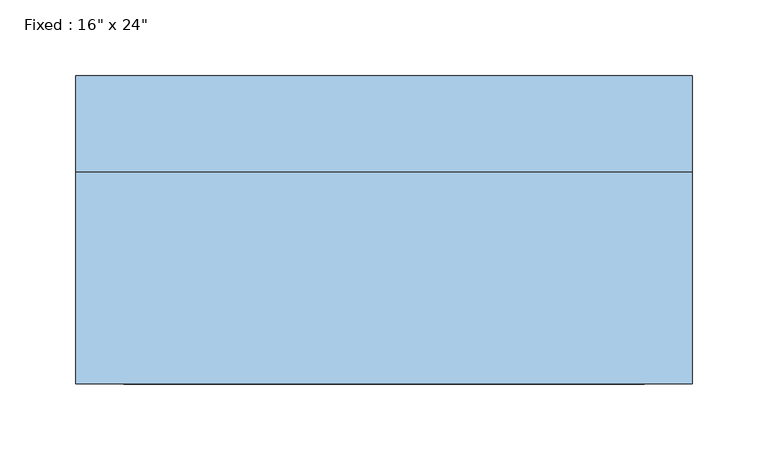
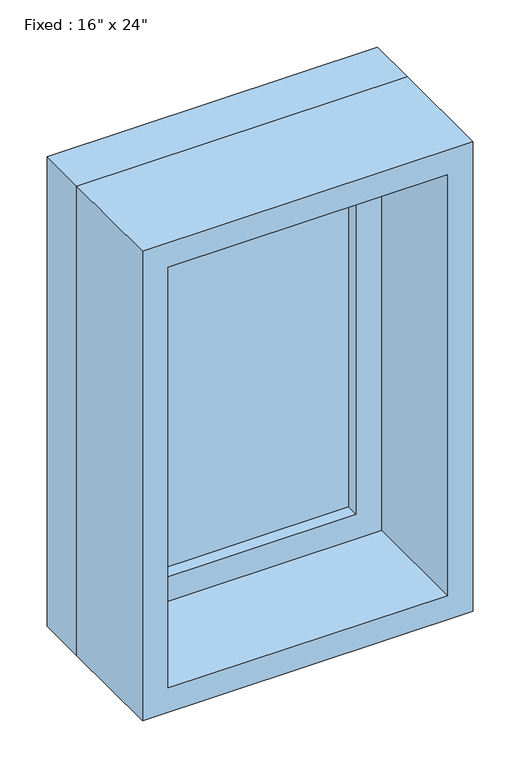
"""IFC4 building model written with IfcOpenShell, lengths in millimetres: window geometry."""

from ifc_helpers import new_model, si_unit, frame, origin, place, context, project, spatial, polyline, outline, extrude, source, transform, mapped, element, save


def window_085f26e1(model_context):
    return source(origin(), model_context, "Body", "SweptSolid", [
        extrude(outline(polyline([(101.6, 53.975), (-177.8, 53.975), (-177.8, 66.675), (101.6, 66.675), (101.6, 53.975)])), frame((0.0, 0.0, 977.9), z_axis=(0.0, 0.0, 1.0), x_axis=(1.0, 0.0, 0.0)), (0.0, 0.0, 1.0), 482.6),
        extrude(outline(polyline([(1504.95, -222.25), (933.45, -222.25), (933.45, 146.05), (1504.95, 146.05), (1504.95, -222.25)]), holes=[polyline([(1460.5, -177.8), (1460.5, 101.6), (977.9, 101.6), (977.9, -177.8), (1460.5, -177.8)])]), frame((0.0, 38.1, 0.0), z_axis=(0.0, 1.0, 0.0), x_axis=(0.0, 0.0, 1.0)), (0.0, 0.0, 1.0), 44.45),
        extrude(outline(polyline([(1524.0, -241.3), (914.4, -241.3), (914.4, 165.1), (1524.0, 165.1), (1524.0, -241.3)]), holes=[polyline([(1492.25, -209.55), (1492.25, 133.35), (946.15, 133.35), (946.15, -209.55), (1492.25, -209.55)])]), frame((0.0, -101.6, 0.0), z_axis=(0.0, 1.0, 0.0), x_axis=(0.0, 0.0, 1.0)), (0.0, 0.0, 1.0), 139.7),
        extrude(outline(polyline([(1524.0, 165.1), (1524.0, -241.3), (914.4, -241.3), (914.4, 165.1), (1524.0, 165.1)]), holes=[polyline([(1504.95, 146.05), (933.45, 146.05), (933.45, -222.25), (1504.95, -222.25), (1504.95, 146.05)])]), frame((0.0, 38.1, 0.0), z_axis=(0.0, 1.0, 0.0), x_axis=(0.0, 0.0, 1.0)), (0.0, 0.0, 1.0), 63.5),
    ])


if __name__ == "__main__":
    model = new_model("IFC4")
    model_context = context("Model", 3, world=origin())
    ifc_project = project(units=[si_unit("LENGTHUNIT", "METRE", prefix="MILLI")], contexts=[model_context])
    site = spatial("IfcSite", under=ifc_project)
    building = spatial("IfcBuilding", under=site)
    placement = place(None, origin())
    window_shape = window_085f26e1(model_context)
    element("IfcWindow", 1, ObjectType="Fixed : 16\" x 24\"", at=placement, inside=building, context=model_context, shape_type="MappedRepresentation", body=[
        mapped(window_shape, transform((0.0, 0.0, 0.0), x_axis=(1.0, 0.0, 0.0), y_axis=(0.0, 1.0, 0.0), z_axis=(0.0, 0.0, 1.0))),
    ])
    save(model, "model.ifc")

# Revit data of these elements
# Type "Fixed : 16\" x 24\""
#   Type Mark = "4"
#   Construction Type Id = "GSP4R"
#   Assembly Code = "B2020100"
#   Analytic Construction = "1/8 in Pilkington single glazing"
#   Visual Light Transmittance = 0.9
#   Solar Heat Gain Coefficient = 0.78
#   Heat Transfer Coefficient (U) = 0.6496 BTU/(h·ft²·°F)
#   Height = 2' - 0"
#   Default Sill Height = 3' - 0"
#   Width = 1' - 4"
#   Window Inset = 0' - 0 3/4"
#   Define Thermal Properties by = 1
#   Glass Pane Material = Glass
#   Sash Material = Sash
#   Wall Closure = (empty or 0)
# Element 1 (IfcWindow, "Fixed : 16\" x 24\"")
#   Materials on its faces: "Sash", "Glass"
# Materials
#   "Glass": class "Glass", colour RGB 0 128 192, transparency 0.75, Description = "Soda Lime Glass", Cost = 0
#   "Sash": class "Wood", colour RGB 224 178 126, transparency 0
